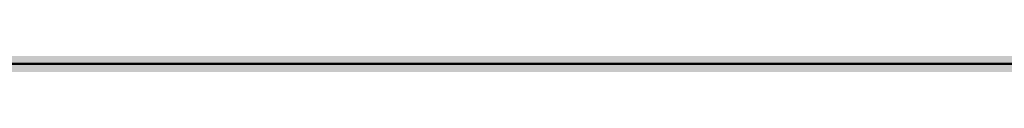
# Model space of a CAD drawing. Units: millimetres. Extents: x 0 to 2267, y 0 to 1823.
# Tile 63 of 256: x 1596.855 to 1600.369, y 1227.247 to 1227.247. Entities that reach past the tile are written whole.
import ezdxf

# ---------------------------------------------------------------- set-up
doc = ezdxf.new("R2010")
doc.units = ezdxf.units.MM
doc.header["$MEASUREMENT"] = 0
doc.layers.add('M-HATC', color=252, linetype='Continuous', lineweight=18)
doc.layers.add('M-OUTL', color=7, linetype='Continuous', lineweight=50)

msp = doc.modelspace()

# ---------------------------------------------------------------- hatches: boundary and pattern name
at = {"layer": 'M-HATC'}
h = msp.add_hatch(color=256, dxfattribs=at)
h.dxf.hatch_style = 1
h.paths.add_polyline_path([(2055.771, 1603.062), (1381.0868, 1603.062), (1381.0868, 1598.062), (2055.771, 1598.062)])
h.paths.add_polyline_path([(2055.771, 1598.062), (1381.0868, 1598.062), (1381.0868, 1593.062), (2055.771, 1593.062)])
h.paths.add_polyline_path([(2051.3074, 1536.7609), (1385.5504, 1536.7609), (1385.5504, 1526.7609), (1387.5504, 1526.7609), (1388.5366, 1525.0528), (1385.3319, 1521.2335), (1385.3319, 1521.2226), (2050.2542, 1522.7491), (2048.3212, 1525.0528), (2049.3074, 1526.7609), (2051.3074, 1526.7609)])
edge = h.paths.add_edge_path()
edge.add_arc((1847.5345, 1379.1492), 135, 222.603061, 222.890851, ccw=False)
edge.add_line((1748.1663, 1287.7656), (1683.0921, 1287.7656))
edge.add_arc((1583.7239, 1379.1492), 135, 317.109149, 317.396939, ccw=False)
edge.add_arc((1678.9686, 1290.6707), 5, 222.8909, 317.1091, ccw=False)
edge.add_arc((1774.2133, 1379.1492), 135, 222.603061, 222.890851, ccw=False)
edge.add_line((1674.8451, 1287.7656), (1609.7709, 1287.7656))
edge.add_arc((1510.4027, 1379.1492), 135, 317.109149, 317.396939, ccw=False)
edge.add_arc((1605.6474, 1290.6707), 5, 222.8909, 317.1091, ccw=False)
edge.add_arc((1700.8921, 1379.1492), 135, 222.603061, 222.890851, ccw=False)
edge.add_line((1601.5239, 1287.7656), (1536.4497, 1287.7656))
edge.add_arc((1437.0815, 1379.1492), 135, 317.109149, 317.396939, ccw=False)
edge.add_arc((1532.3262, 1290.6707), 5, 222.8909, 317.1091, ccw=False)
edge.add_arc((1627.5709, 1379.1492), 135, 222.603061, 222.890851, ccw=False)
edge.add_line((1528.2027, 1287.7656), (1505.9289, 1287.7656))
edge.add_spline(control_points=[(1505.9289, 1287.7656), (1504.2622, 1287.7656), (1504.2622, 1282.7656), (1505.9289, 1282.7656)], knot_values=[0, 0, 0, 0, 5, 5, 5, 5], degree=3, periodic=0)
edge.add_line((1505.9289, 1282.7656), (1930.9289, 1282.7656))
edge.add_spline(control_points=[(1930.9289, 1282.7656), (1932.5956, 1282.7656), (1932.5956, 1287.7656), (1930.9289, 1287.7656)], knot_values=[0, 0, 0, 0, 5, 5, 5, 5], degree=3, periodic=0)
edge.add_line((1930.9289, 1287.7656), (1903.0557, 1287.7656))
edge.add_arc((1803.6875, 1379.1492), 135, 317.109149, 317.396939, ccw=False)
edge.add_arc((1898.9322, 1290.6707), 5, 222.8909, 317.1091, ccw=False)
edge.add_arc((1994.1769, 1379.1492), 135, 222.603061, 222.890851, ccw=False)
edge.add_line((1894.8087, 1287.7656), (1829.7345, 1287.7656))
edge.add_arc((1730.3663, 1379.1492), 135, 317.109149, 317.396939, ccw=False)
edge.add_arc((1825.611, 1290.6707), 5, 222.8909, 317.1091, ccw=False)
edge.add_arc((1920.8557, 1379.1492), 135, 222.603061, 222.890851, ccw=False)
edge.add_line((1821.4875, 1287.7656), (1756.4133, 1287.7656))
edge.add_arc((1657.0451, 1379.1492), 135, 317.109149, 317.396939, ccw=False)
edge.add_arc((1752.2898, 1290.6707), 5, 222.8909, 317.1091, ccw=False)
edge = h.paths.add_edge_path()
edge.add_spline(control_points=[(1843.4289, 1227.2475), (1845.0956, 1227.2475), (1845.0956, 1232.2475), (1843.4289, 1232.2475)], knot_values=[0, 0, 0, 0, 5, 5, 5, 5], degree=3, periodic=0)
edge.add_line((1843.4289, 1232.2475), (1593.4289, 1232.2475))
edge.add_spline(control_points=[(1593.4289, 1232.2475), (1591.7622, 1232.2475), (1591.7622, 1227.2475), (1593.4289, 1227.2475)], knot_values=[0, 0, 0, 0, 5, 5, 5, 5], degree=3, periodic=0)
edge.add_line((1593.4289, 1227.2475), (1843.4289, 1227.2475))
h.paths.add_polyline_path([(1905.9289, 1127.4171), (1530.9289, 1127.4171, 0.414214), (1520.9289, 1117.4171), (1530.9289, 1117.4171), (1915.9289, 1117.4171, 0.414214)])
edge = h.paths.add_edge_path()
edge.add_arc((1397.0858, 1498.4078), 12.7299, 90.78215, 190.87871, ccw=False)
edge.add_line((1396.912, 1511.1365), (1428.0097, 1511.3488))
edge.add_line((1428.0097, 1511.3488), (1433.0097, 1511.3488))
edge.add_line((1433.0097, 1511.3488), (1434.439, 1511.3488))
edge.add_arc((1419.474, 1498.0804), 20, 41.561, 74.08211)
edge.add_line((1424.9592, 1517.3135), (1399.9351, 1517.2561))
edge.add_spline(control_points=[(1399.9307, 1517.2561), (1399.884, 1517.2131), (1399.8328, 1517.1689), (1399.7774, 1517.1236)], knot_values=[11.567499, 11.567499, 11.567499, 11.567499, 11.814249, 11.814249, 11.814249, 11.814249], degree=3, periodic=0)
edge.add_spline(control_points=[(1399.6328, 1517.0099), (1399.5831, 1516.9721), (1399.5307, 1516.9338), (1399.4759, 1516.8947)], knot_values=[11.167718, 11.167718, 11.167718, 11.167718, 11.365188, 11.365188, 11.365188, 11.365188], degree=3, periodic=0)
edge.add_spline(control_points=[(1399.3398, 1516.8001), (1399.1514, 1516.6719), (1398.9384, 1516.5377), (1398.704, 1516.3994)], knot_values=[10.376405, 10.376405, 10.376405, 10.376405, 11.00994, 11.00994, 11.00994, 11.00994], degree=3, periodic=0)
edge.add_spline(control_points=[(1398.6572, 1516.3719), (1398.5789, 1516.326), (1398.4983, 1516.2797), (1398.4155, 1516.2331)], knot_values=[10.125175, 10.125175, 10.125175, 10.125175, 10.334406, 10.334406, 10.334406, 10.334406], degree=3, periodic=0)
edge.add_spline(control_points=[(1398.2642, 1516.1487), (1398.196, 1516.1111), (1398.1263, 1516.0732), (1398.0555, 1516.0351)], knot_values=[9.832246, 9.832246, 9.832246, 9.832246, 9.999658, 9.999658, 9.999658, 9.999658], degree=3, periodic=0)
edge.add_spline(control_points=[(1397.9987, 1516.0048), (1397.7312, 1515.8621), (1397.446, 1515.7171), (1397.1466, 1515.5714)], knot_values=[9.161808, 9.161808, 9.161808, 9.161808, 9.787769, 9.787769, 9.787769, 9.787769], degree=3, periodic=0)
edge.add_spline(control_points=[(1397.1466, 1515.5714), (1396.8418, 1515.423), (1396.5222, 1515.274), (1396.1914, 1515.1262)], knot_values=[8.524455, 8.524455, 8.524455, 8.524455, 9.161808, 9.161808, 9.161808, 9.161808], degree=3, periodic=0)
edge.add_spline(control_points=[(1396.0777, 1515.0756), (1395.9854, 1515.0348), (1395.8922, 1514.994), (1395.7983, 1514.9534)], knot_values=[8.275193, 8.275193, 8.275193, 8.275193, 8.451726, 8.451726, 8.451726, 8.451726], degree=3, periodic=0)
edge.add_spline(control_points=[(1395.6018, 1514.8691), (1395.4997, 1514.8257), (1395.3968, 1514.7824), (1395.2932, 1514.7394)], knot_values=[7.962917, 7.962917, 7.962917, 7.962917, 8.152764, 8.152764, 8.152764, 8.152764], degree=3, periodic=0)
edge.add_spline(control_points=[(1395.2116, 1514.7057), (1394.8278, 1514.5475), (1394.4345, 1514.3929), (1394.0364, 1514.2442)], knot_values=[7.21254, 7.21254, 7.21254, 7.21254, 7.913148, 7.913148, 7.913148, 7.913148], degree=3, periodic=0)
edge.add_spline(control_points=[(1394.0364, 1514.2442), (1393.7076, 1514.1214), (1393.3754, 1514.0027), (1393.0427, 1513.8895)], knot_values=[6.633733, 6.633733, 6.633733, 6.633733, 7.21254, 7.21254, 7.21254, 7.21254], degree=3, periodic=0)
edge.add_spline(control_points=[(1392.8214, 1513.815), (1392.7198, 1513.7812), (1392.6181, 1513.7479), (1392.5166, 1513.7152)], knot_values=[6.328796, 6.328796, 6.328796, 6.328796, 6.505493, 6.505493, 6.505493, 6.505493], degree=3, periodic=0)
edge.add_spline(control_points=[(1392.5166, 1513.7152), (1392.3187, 1513.6515), (1392.1212, 1513.59), (1391.9244, 1513.531)], knot_values=[5.984605, 5.984605, 5.984605, 5.984605, 6.328796, 6.328796, 6.328796, 6.328796], degree=3, periodic=0)
edge.add_spline(control_points=[(1391.7915, 1513.4915), (1391.3122, 1513.3501), (1390.8384, 1513.2239), (1390.3784, 1513.1171)], knot_values=[5.066697, 5.066697, 5.066697, 5.066697, 5.907055, 5.907055, 5.907055, 5.907055], degree=3, periodic=0)
edge.add_spline(control_points=[(1390.3784, 1513.1171), (1390.1797, 1513.071), (1389.9836, 1513.0284), (1389.7907, 1512.9899)], knot_values=[4.70367, 4.70367, 4.70367, 4.70367, 5.066695, 5.066695, 5.066695, 5.066695], degree=3, periodic=0)
edge.add_spline(control_points=[(1389.422, 1512.9204), (1389.2459, 1512.8892), (1389.0729, 1512.8617), (1388.9036, 1512.8381)], knot_values=[4.130571, 4.130571, 4.130571, 4.130571, 4.469816, 4.469816, 4.469816, 4.469816], degree=3, periodic=0)
edge.add_spline(control_points=[(1388.9036, 1512.8381), (1388.591, 1512.7946), (1388.2911, 1512.7644), (1388.0071, 1512.7494)], knot_values=[3.504031, 3.504031, 3.504031, 3.504031, 4.130571, 4.130571, 4.130571, 4.130571], degree=3, periodic=0)
edge.add_spline(control_points=[(1387.9356, 1512.7459), (1387.8538, 1512.7423), (1387.7733, 1512.74), (1387.6944, 1512.739)], knot_values=[3.268866, 3.268866, 3.268866, 3.268866, 3.451164, 3.451164, 3.451164, 3.451164], degree=3, periodic=0)
edge.add_spline(control_points=[(1387.3351, 1512.7443), (1387.2076, 1512.7499), (1387.0847, 1512.7597), (1386.967, 1512.7739)], knot_values=[2.670686, 2.670686, 2.670686, 2.670686, 2.984, 2.984, 2.984, 2.984], degree=3, periodic=0)
edge.add_spline(control_points=[(1386.8327, 1512.7922), (1386.8209, 1512.7941), (1386.8092, 1512.7959), (1386.7975, 1512.7979)], knot_values=[2.516981, 2.516981, 2.516981, 2.516981, 2.549528, 2.549528, 2.549528, 2.549528], degree=3, periodic=0)
edge.add_spline(control_points=[(1386.4526, 1512.8735), (1386.4257, 1512.881), (1386.3993, 1512.889), (1386.3733, 1512.8972)], knot_values=[2.095869, 2.095869, 2.095869, 2.095869, 2.17941, 2.17941, 2.17941, 2.17941], degree=3, periodic=0)
edge.add_spline(control_points=[(1386.0691, 1513.0189), (1386.0634, 1513.0217), (1386.0577, 1513.0246), (1386.052, 1513.0275)], knot_values=[1.72453, 1.72453, 1.72453, 1.72453, 1.745933, 1.745933, 1.745933, 1.745933], degree=3, periodic=0)
edge.add_arc((1399.474, 1498.0804), 20, 131.82432, 180)
edge.add_arc((1630.3336, 1505.5484), 250.9708, 181.705176, 236.427975)
edge.add_arc((1605.3399, 1483.3044), 218.7822, 238.660829, 243.34961)
edge.add_arc((1647.0911, 1510.3592), 262.8986, 183.129836, 237.853442, ccw=False)
h.paths.add_polyline_path([(1406.5369, 1391.9644, 0.149382), (1491.5506, 1296.4418, -0.129517)], flags=17)
edge = h.paths.add_edge_path()
edge.add_arc((2037.3838, 1498.0804), 20, 0, 48.26587)
edge.add_spline(control_points=[(2050.6973, 1513.0052), (2050.6512, 1512.9847), (2050.6034, 1512.9655), (2050.5539, 1512.9477)], knot_values=[1.835652, 1.835652, 1.835652, 1.835652, 2.000781, 2.000781, 2.000781, 2.000781], degree=3, periodic=0)
edge.add_spline(control_points=[(2050.4616, 1512.9166), (2050.479, 1512.9221), (2050.4963, 1512.9277), (2050.5133, 1512.9335)], knot_values=[2.045477, 2.045477, 2.045477, 2.045477, 2.101389, 2.101389, 2.101389, 2.101389], degree=3, periodic=0)
edge.add_spline(control_points=[(2050.129, 1512.8342), (2050.1984, 1512.8473), (2050.2657, 1512.8623), (2050.3308, 1512.8792)], knot_values=[2.237629, 2.237629, 2.237629, 2.237629, 2.435841, 2.435841, 2.435841, 2.435841], degree=3, periodic=0)
edge.add_spline(control_points=[(2050.0946, 1512.8278), (2050.1061, 1512.8299), (2050.1176, 1512.832), (2050.129, 1512.8342)], knot_values=[2.435841, 2.435841, 2.435841, 2.435841, 2.468321, 2.468321, 2.468321, 2.468321], degree=3, periodic=0)
edge.add_spline(control_points=[(2049.7843, 1512.7851), (2049.8552, 1512.7922), (2049.9243, 1512.8008), (2049.9917, 1512.8109)], knot_values=[2.563852, 2.563852, 2.563852, 2.563852, 2.748541, 2.748541, 2.748541, 2.748541], degree=3, periodic=0)
edge.add_spline(control_points=[(2049.4052, 1512.7617), (2049.5364, 1512.7653), (2049.6629, 1512.773), (2049.7843, 1512.7851)], knot_values=[2.748541, 2.748541, 2.748541, 2.748541, 3.064882, 3.064882, 3.064882, 3.064882], degree=3, periodic=0)
edge.add_spline(control_points=[(2049.1698, 1512.7597), (2049.2336, 1512.7591), (2049.2965, 1512.7594), (2049.3584, 1512.7606)], knot_values=[3.102309, 3.102309, 3.102309, 3.102309, 3.2503, 3.2503, 3.2503, 3.2503], degree=3, periodic=0)
edge.add_spline(control_points=[(2048.8573, 1512.7691), (2048.9638, 1512.7638), (2049.068, 1512.7606), (2049.1698, 1512.7597)], knot_values=[3.2503, 3.2503, 3.2503, 3.2503, 3.486069, 3.486069, 3.486069, 3.486069], degree=3, periodic=0)
edge.add_spline(control_points=[(2048.6924, 1512.7789), (2048.3729, 1512.8009), (2048.0345, 1512.8411), (2047.6817, 1512.897)], knot_values=[3.606429, 3.606429, 3.606429, 3.606429, 4.2989, 4.2989, 4.2989, 4.2989], degree=3, periodic=0)
edge.add_spline(control_points=[(2047.6817, 1512.897), (2047.5458, 1512.9185), (2047.4077, 1512.9424), (2047.2678, 1512.9685)], knot_values=[4.2989, 4.2989, 4.2989, 4.2989, 4.565769, 4.565769, 4.565769, 4.565769], degree=3, periodic=0)
edge.add_spline(control_points=[(2047.2678, 1512.9685), (2047.1449, 1512.9914), (2047.0207, 1513.016), (2046.8951, 1513.0422)], knot_values=[4.565769, 4.565769, 4.565769, 4.565769, 4.799971, 4.799971, 4.799971, 4.799971], degree=3, periodic=0)
edge.add_spline(control_points=[(2046.8951, 1513.0422), (2046.5286, 1513.1188), (2046.1513, 1513.209), (2045.7676, 1513.3107)], knot_values=[4.799971, 4.799971, 4.799971, 4.799971, 5.483718, 5.483718, 5.483718, 5.483718], degree=3, periodic=0)
edge.add_spline(control_points=[(2045.7676, 1513.3107), (2045.3724, 1513.4154), (2044.9704, 1513.5322), (2044.5662, 1513.6588)], knot_values=[5.483718, 5.483718, 5.483718, 5.483718, 6.187866, 6.187866, 6.187866, 6.187866], degree=3, periodic=0)
edge.add_spline(control_points=[(2044.5662, 1513.6588), (2044.4149, 1513.7061), (2044.2633, 1513.7549), (2044.1116, 1513.8048)], knot_values=[6.187866, 6.187866, 6.187866, 6.187866, 6.451551, 6.451551, 6.451551, 6.451551], degree=3, periodic=0)
edge.add_spline(control_points=[(2044.1116, 1513.8048), (2043.9967, 1513.8427), (2043.8817, 1513.8813), (2043.7668, 1513.9205)], knot_values=[6.451551, 6.451551, 6.451551, 6.451551, 6.651434, 6.651434, 6.651434, 6.651434], degree=3, periodic=0)
edge.add_spline(control_points=[(2043.7668, 1513.9205), (2043.3716, 1514.0554), (2042.9774, 1514.1979), (2042.5886, 1514.3458)], knot_values=[6.651434, 6.651434, 6.651434, 6.651434, 7.338879, 7.338879, 7.338879, 7.338879], degree=3, periodic=0)
edge.add_spline(control_points=[(2042.5886, 1514.3458), (2042.1643, 1514.5071), (2041.7465, 1514.6749), (2041.3409, 1514.846)], knot_values=[7.338879, 7.338879, 7.338879, 7.338879, 8.089209, 8.089209, 8.089209, 8.089209], degree=3, periodic=0)
edge.add_spline(control_points=[(2041.3409, 1514.846), (2041.1028, 1514.9465), (2040.869, 1515.0481), (2040.6405, 1515.1502)], knot_values=[8.089209, 8.089209, 8.089209, 8.089209, 8.529587, 8.529587, 8.529587, 8.529587], degree=3, periodic=0)
edge.add_spline(control_points=[(2040.51, 1515.2089), (2040.0824, 1515.4022), (2039.6747, 1515.5971), (2039.295, 1515.7894)], knot_values=[8.613818, 8.613818, 8.613818, 8.613818, 9.44571, 9.44571, 9.44571, 9.44571], degree=3, periodic=0)
edge.add_spline(control_points=[(2039.295, 1515.7894), (2039.0618, 1515.9075), (2038.8391, 1516.0246), (2038.6288, 1516.1398)], knot_values=[9.44571, 9.44571, 9.44571, 9.44571, 9.956404, 9.956404, 9.956404, 9.956404], degree=3, periodic=0)
edge.add_spline(control_points=[(2038.6288, 1516.1398), (2038.5187, 1516.2001), (2038.4121, 1516.2598), (2038.309, 1516.3189)], knot_values=[9.956404, 9.956404, 9.956404, 9.956404, 10.223542, 10.223542, 10.223542, 10.223542], degree=3, periodic=0)
edge.add_spline(control_points=[(2038.309, 1516.3189), (2038.2138, 1516.3735), (2038.1216, 1516.4276), (2038.0328, 1516.481)], knot_values=[10.223542, 10.223542, 10.223542, 10.223542, 10.47051, 10.47051, 10.47051, 10.47051], degree=3, periodic=0)
edge.add_spline(control_points=[(2038.0328, 1516.481), (2037.7855, 1516.6296), (2037.5639, 1516.773), (2037.3722, 1516.909)], knot_values=[10.47051, 10.47051, 10.47051, 10.47051, 11.15767, 11.15767, 11.15767, 11.15767], degree=3, periodic=0)
edge.add_spline(control_points=[(2037.3722, 1516.909), (2037.2789, 1516.9752), (2037.1927, 1517.0396), (2037.1142, 1517.102)], knot_values=[11.15767, 11.15767, 11.15767, 11.15767, 11.49227, 11.49227, 11.49227, 11.49227], degree=3, periodic=0)
edge.add_spline(control_points=[(2036.8564, 1517.3259), (2036.9148, 1517.2692), (2036.9814, 1517.2103), (2037.0557, 1517.1492)], knot_values=[11.577341, 11.577341, 11.577341, 11.577341, 11.91035, 11.91035, 11.91035, 11.91035], degree=3, periodic=0)
edge.add_spline(control_points=[(2036.8074, 1517.3748), (2036.823, 1517.3587), (2036.8393, 1517.3424), (2036.8564, 1517.3259)], knot_values=[11.91035, 11.91035, 11.91035, 11.91035, 12.007402, 12.007402, 12.007402, 12.007402], degree=3, periodic=0)
edge.add_spline(control_points=[(2036.7017, 1517.494), (2036.7104, 1517.483), (2036.7196, 1517.4719), (2036.7291, 1517.4606)], knot_values=[12.184155, 12.184155, 12.184155, 12.184155, 12.255409, 12.255409, 12.255409, 12.255409], degree=3, periodic=0)
edge.add_spline(control_points=[(2036.6159, 1517.6205), (2036.62, 1517.613), (2036.6243, 1517.6055), (2036.6289, 1517.5979)], knot_values=[12.487913, 12.487913, 12.487913, 12.487913, 12.541035, 12.541035, 12.541035, 12.541035], degree=3, periodic=0)
edge.add_spline(control_points=[(2036.5635, 1517.786), (2036.5637, 1517.7794), (2036.5642, 1517.7726), (2036.565, 1517.7658)], knot_values=[12.911761, 12.911761, 12.911761, 12.911761, 12.968286, 12.968286, 12.968286, 12.968286], degree=3, periodic=0)
edge.add_spline(control_points=[(2036.6166, 1517.9304), (2036.6125, 1517.9259), (2036.6086, 1517.9212), (2036.6049, 1517.9165)], knot_values=[13.382527, 13.382527, 13.382527, 13.382527, 13.433791, 13.433791, 13.433791, 13.433791], degree=3, periodic=0)
edge.add_spline(control_points=[(2036.749, 1518.017), (2036.7361, 1518.0116), (2036.7239, 1518.006), (2036.7124, 1518.0002)], knot_values=[13.726299, 13.726299, 13.726299, 13.726299, 13.809928, 13.809928, 13.809928, 13.809928], degree=3, periodic=0)
edge.add_spline(control_points=[(2036.8604, 1518.0528), (2036.8386, 1518.0474), (2036.8181, 1518.0416), (2036.7988, 1518.0353)], knot_values=[13.910887, 13.910887, 13.910887, 13.910887, 14.02153, 14.02153, 14.02153, 14.02153], degree=3, periodic=0)
edge.add_line((2036.9639, 1518.0804), (2032.3838, 1518.0804))
edge.add_line((2032.3838, 1518.0804), (2027.3838, 1518.0804))
edge.add_line((2027.3838, 1518.0804), (2022.3838, 1518.0804))
edge.add_line((2022.3838, 1518.0804), (2017.3838, 1518.0804))
edge.add_arc((2017.3838, 1498.0804), 20, 90, 138.439)
edge.add_line((2002.4188, 1511.3488), (2003.8481, 1511.3488))
edge.add_line((2003.8481, 1511.3488), (2008.8481, 1511.3488))
edge.add_line((2008.8481, 1511.3488), (2039.772, 1511.1377))
edge.add_arc((2039.772, 1498.4078), 12.7299, -10.87871, 90, ccw=False)
edge.add_arc((1789.7668, 1510.3592), 262.8986, 302.146558, 356.870164, ccw=False)
edge.add_arc((1831.5179, 1483.3044), 218.7822, 296.65039, 301.339171)
edge.add_arc((1806.5242, 1505.5484), 250.9708, 303.572025, 358.294824)
h.paths.add_polyline_path([(2030.321, 1391.9644, -0.129517), (1945.3072, 1296.4418, 0.149382)], flags=17)
edge = h.paths.add_edge_path()
edge.add_spline(control_points=[(2037.2464, 1518.0821), (2037.2898, 1518.081), (2037.3355, 1518.0804), (2037.3838, 1518.0804)], knot_values=[0.000012, 0.000012, 0.000012, 0.000012, 0.144754, 0.144754, 0.144754, 0.144754], degree=3, periodic=0)
edge.add_line((2037.3357, 1518.0804), (2037.0096, 1518.0804))
edge.add_spline(control_points=[(2037.0096, 1518.0804), (2036.9822, 1518.0768), (2036.956, 1518.0727), (2036.9312, 1518.0681)], knot_values=[14.13465, 14.13465, 14.13465, 14.13465, 14.247197, 14.247197, 14.247197, 14.247197], degree=3, periodic=0)
edge.add_spline(control_points=[(2036.9312, 1518.0681), (2036.9276, 1518.0674), (2036.9241, 1518.0667), (2036.9205, 1518.0661)], knot_values=[14.118315, 14.118315, 14.118315, 14.118315, 14.13465, 14.13465, 14.13465, 14.13465], degree=3, periodic=0)
edge.add_spline(control_points=[(2036.9205, 1518.0661), (2036.9118, 1518.0644), (2036.9032, 1518.0626), (2036.8948, 1518.0608)], knot_values=[14.078086, 14.078086, 14.078086, 14.078086, 14.118315, 14.118315, 14.118315, 14.118315], degree=3, periodic=0)
edge.add_spline(control_points=[(2036.8948, 1518.0608), (2036.883, 1518.0583), (2036.8716, 1518.0556), (2036.8604, 1518.0528)], knot_values=[14.02153, 14.02153, 14.02153, 14.02153, 14.078086, 14.078086, 14.078086, 14.078086], degree=3, periodic=0)
edge.add_spline(control_points=[(2036.8604, 1518.0528), (2036.8386, 1518.0474), (2036.8181, 1518.0416), (2036.7988, 1518.0353)], knot_values=[13.910887, 13.910887, 13.910887, 13.910887, 14.02153, 14.02153, 14.02153, 14.02153], degree=3, periodic=0)
edge.add_spline(control_points=[(2036.7988, 1518.0353), (2036.7981, 1518.035), (2036.7974, 1518.0348), (2036.7967, 1518.0346)], knot_values=[13.906906, 13.906906, 13.906906, 13.906906, 13.910887, 13.910887, 13.910887, 13.910887], degree=3, periodic=0)
edge.add_spline(control_points=[(2036.7967, 1518.0346), (2036.7882, 1518.0318), (2036.7799, 1518.0289), (2036.7719, 1518.0259)], knot_values=[13.857826, 13.857826, 13.857826, 13.857826, 13.906906, 13.906906, 13.906906, 13.906906], degree=3, periodic=0)
edge.add_spline(control_points=[(2036.7719, 1518.0259), (2036.764, 1518.023), (2036.7564, 1518.02), (2036.749, 1518.017)], knot_values=[13.809928, 13.809928, 13.809928, 13.809928, 13.857826, 13.857826, 13.857826, 13.857826], degree=3, periodic=0)
edge.add_spline(control_points=[(2036.749, 1518.017), (2036.7361, 1518.0116), (2036.7239, 1518.006), (2036.7124, 1518.0002)], knot_values=[13.726299, 13.726299, 13.726299, 13.726299, 13.809928, 13.809928, 13.809928, 13.809928], degree=3, periodic=0)
edge.add_spline(control_points=[(2036.7124, 1518.0002), (2036.7121, 1518), (2036.7118, 1517.9999), (2036.7115, 1517.9997)], knot_values=[13.723993, 13.723993, 13.723993, 13.723993, 13.726299, 13.726299, 13.726299, 13.726299], degree=3, periodic=0)
edge.add_spline(control_points=[(2036.7115, 1517.9997), (2036.7063, 1517.9971), (2036.7013, 1517.9944), (2036.6965, 1517.9917)], knot_values=[13.686536, 13.686536, 13.686536, 13.686536, 13.723993, 13.723993, 13.723993, 13.723993], degree=3, periodic=0)
edge.add_spline(control_points=[(2036.6965, 1517.9917), (2036.6919, 1517.9891), (2036.6874, 1517.9865), (2036.6831, 1517.9839)], knot_values=[13.651251, 13.651251, 13.651251, 13.651251, 13.686536, 13.686536, 13.686536, 13.686536], degree=3, periodic=0)
edge.add_spline(control_points=[(2036.6831, 1517.9839), (2036.6764, 1517.9798), (2036.67, 1517.9757), (2036.6639, 1517.9714)], knot_values=[13.596804, 13.596804, 13.596804, 13.596804, 13.651251, 13.651251, 13.651251, 13.651251], degree=3, periodic=0)
edge.add_spline(control_points=[(2036.6639, 1517.9714), (2036.6636, 1517.9712), (2036.6633, 1517.9709), (2036.6629, 1517.9707)], knot_values=[13.593956, 13.593956, 13.593956, 13.593956, 13.596804, 13.596804, 13.596804, 13.596804], degree=3, periodic=0)
edge.add_spline(control_points=[(2036.6629, 1517.9707), (2036.6603, 1517.9689), (2036.6577, 1517.967), (2036.6552, 1517.9651)], knot_values=[13.570322, 13.570322, 13.570322, 13.570322, 13.593956, 13.593956, 13.593956, 13.593956], degree=3, periodic=0)
edge.add_spline(control_points=[(2036.6552, 1517.9651), (2036.6525, 1517.9631), (2036.6499, 1517.9611), (2036.6474, 1517.9591)], knot_values=[13.545477, 13.545477, 13.545477, 13.545477, 13.570322, 13.570322, 13.570322, 13.570322], degree=3, periodic=0)
edge.add_spline(control_points=[(2036.6474, 1517.9591), (2036.6472, 1517.9589), (2036.6471, 1517.9588), (2036.6469, 1517.9587)], knot_values=[13.543931, 13.543931, 13.543931, 13.543931, 13.545477, 13.545477, 13.545477, 13.545477], degree=3, periodic=0)
edge.add_spline(control_points=[(2036.6469, 1517.9587), (2036.6412, 1517.9541), (2036.6358, 1517.9494), (2036.6307, 1517.9447)], knot_values=[13.488237, 13.488237, 13.488237, 13.488237, 13.543931, 13.543931, 13.543931, 13.543931], degree=3, periodic=0)
edge.add_spline(control_points=[(2036.6307, 1517.9447), (2036.6282, 1517.9423), (2036.6257, 1517.9399), (2036.6233, 1517.9374)], knot_values=[13.460307, 13.460307, 13.460307, 13.460307, 13.488237, 13.488237, 13.488237, 13.488237], degree=3, periodic=0)
edge.add_spline(control_points=[(2036.6233, 1517.9374), (2036.6215, 1517.9356), (2036.6198, 1517.9338), (2036.6181, 1517.932)], knot_values=[13.439712, 13.439712, 13.439712, 13.439712, 13.460307, 13.460307, 13.460307, 13.460307], degree=3, periodic=0)
edge.add_spline(control_points=[(2036.6181, 1517.932), (2036.6176, 1517.9315), (2036.6171, 1517.9309), (2036.6166, 1517.9304)], knot_values=[13.433791, 13.433791, 13.433791, 13.433791, 13.439712, 13.439712, 13.439712, 13.439712], degree=3, periodic=0)
edge.add_spline(control_points=[(2036.6166, 1517.9304), (2036.6125, 1517.9259), (2036.6086, 1517.9212), (2036.6049, 1517.9165)], knot_values=[13.382527, 13.382527, 13.382527, 13.382527, 13.433791, 13.433791, 13.433791, 13.433791], degree=3, periodic=0)
edge.add_spline(control_points=[(2036.6049, 1517.9165), (2036.6026, 1517.9135), (2036.6004, 1517.9104), (2036.5982, 1517.9074)], knot_values=[13.350017, 13.350017, 13.350017, 13.350017, 13.382527, 13.382527, 13.382527, 13.382527], degree=3, periodic=0)
edge.add_spline(control_points=[(2036.5982, 1517.9074), (2036.5972, 1517.9059), (2036.5962, 1517.9043), (2036.5952, 1517.9028)], knot_values=[13.333922, 13.333922, 13.333922, 13.333922, 13.350017, 13.350017, 13.350017, 13.350017], degree=3, periodic=0)
edge.add_spline(control_points=[(2036.5952, 1517.9028), (2036.5945, 1517.9018), (2036.5939, 1517.9009), (2036.5933, 1517.8999)], knot_values=[13.323828, 13.323828, 13.323828, 13.323828, 13.333922, 13.333922, 13.333922, 13.333922], degree=3, periodic=0)
edge.add_spline(control_points=[(2036.5933, 1517.8999), (2036.5905, 1517.8955), (2036.5879, 1517.8909), (2036.5855, 1517.8864)], knot_values=[13.277545, 13.277545, 13.277545, 13.277545, 13.323828, 13.323828, 13.323828, 13.323828], degree=3, periodic=0)
edge.add_spline(control_points=[(2036.5855, 1517.8864), (2036.5836, 1517.8827), (2036.5817, 1517.8789), (2036.5801, 1517.8751)], knot_values=[13.240119, 13.240119, 13.240119, 13.240119, 13.277545, 13.277545, 13.277545, 13.277545], degree=3, periodic=0)
edge.add_spline(control_points=[(2036.5801, 1517.8751), (2036.5795, 1517.8739), (2036.579, 1517.8727), (2036.5785, 1517.8715)], knot_values=[13.228211, 13.228211, 13.228211, 13.228211, 13.240119, 13.240119, 13.240119, 13.240119], degree=3, periodic=0)
edge.add_spline(control_points=[(2036.5785, 1517.8715), (2036.578, 1517.8702), (2036.5774, 1517.869), (2036.5769, 1517.8677)], knot_values=[13.215717, 13.215717, 13.215717, 13.215717, 13.228211, 13.228211, 13.228211, 13.228211], degree=3, periodic=0)
edge.add_spline(control_points=[(2036.5769, 1517.8677), (2036.5755, 1517.864), (2036.5741, 1517.8603), (2036.5729, 1517.8565)], knot_values=[13.179847, 13.179847, 13.179847, 13.179847, 13.215717, 13.215717, 13.215717, 13.215717], degree=3, periodic=0)
edge.add_spline(control_points=[(2036.5729, 1517.8565), (2036.5713, 1517.8515), (2036.5699, 1517.8464), (2036.5687, 1517.8413)], knot_values=[13.132017, 13.132017, 13.132017, 13.132017, 13.179847, 13.179847, 13.179847, 13.179847], degree=3, periodic=0)
edge.add_spline(control_points=[(2036.5687, 1517.8413), (2036.5684, 1517.8402), (2036.5682, 1517.8392), (2036.568, 1517.8382)], knot_values=[13.122482, 13.122482, 13.122482, 13.122482, 13.132017, 13.132017, 13.132017, 13.132017], degree=3, periodic=0)
edge.add_spline(control_points=[(2036.568, 1517.8382), (2036.5676, 1517.8363), (2036.5672, 1517.8345), (2036.5669, 1517.8327)], knot_values=[13.105592, 13.105592, 13.105592, 13.105592, 13.122482, 13.122482, 13.122482, 13.122482], degree=3, periodic=0)
edge.add_spline(control_points=[(2036.5669, 1517.8327), (2036.5662, 1517.8292), (2036.5657, 1517.8257), (2036.5652, 1517.8222)], knot_values=[13.074063, 13.074063, 13.074063, 13.074063, 13.105592, 13.105592, 13.105592, 13.105592], degree=3, periodic=0)
edge.add_spline(control_points=[(2036.5652, 1517.8222), (2036.5652, 1517.8222), (2036.5652, 1517.8222), (2036.5652, 1517.8222)], knot_values=[13.074043, 13.074043, 13.074043, 13.074043, 13.074063, 13.074063, 13.074063, 13.074063], degree=3, periodic=0)
edge.add_spline(control_points=[(2036.5652, 1517.8222), (2036.5644, 1517.8164), (2036.5639, 1517.8106), (2036.5636, 1517.8046)], knot_values=[13.021884, 13.021884, 13.021884, 13.021884, 13.074043, 13.074043, 13.074043, 13.074043], degree=3, periodic=0)
edge.add_spline(control_points=[(2036.5636, 1517.8046), (2036.5636, 1517.804), (2036.5636, 1517.8034), (2036.5635, 1517.8028)], knot_values=[13.01674, 13.01674, 13.01674, 13.01674, 13.021884, 13.021884, 13.021884, 13.021884], degree=3, periodic=0)
edge.add_spline(control_points=[(2036.5635, 1517.8028), (2036.5634, 1517.8005), (2036.5634, 1517.7982), (2036.5634, 1517.7958)], knot_values=[12.996438, 12.996438, 12.996438, 12.996438, 13.01674, 13.01674, 13.01674, 13.01674], degree=3, periodic=0)
edge.add_spline(control_points=[(2036.5634, 1517.7958), (2036.5633, 1517.7926), (2036.5634, 1517.7893), (2036.5635, 1517.786)], knot_values=[12.968286, 12.968286, 12.968286, 12.968286, 12.996438, 12.996438, 12.996438, 12.996438], degree=3, periodic=0)
edge.add_spline(control_points=[(2036.5635, 1517.786), (2036.5637, 1517.7794), (2036.5642, 1517.7726), (2036.565, 1517.7658)], knot_values=[12.911761, 12.911761, 12.911761, 12.911761, 12.968286, 12.968286, 12.968286, 12.968286], degree=3, periodic=0)
edge.add_spline(control_points=[(2036.565, 1517.7658), (2036.565, 1517.7657), (2036.565, 1517.7656), (2036.565, 1517.7656)], knot_values=[12.911017, 12.911017, 12.911017, 12.911017, 12.911761, 12.911761, 12.911761, 12.911761], degree=3, periodic=0)
edge.add_spline(control_points=[(2036.565, 1517.7656), (2036.5654, 1517.7625), (2036.5658, 1517.7593), (2036.5663, 1517.7562)], knot_values=[12.88528, 12.88528, 12.88528, 12.88528, 12.911017, 12.911017, 12.911017, 12.911017], degree=3, periodic=0)
edge.add_spline(control_points=[(2036.5663, 1517.7562), (2036.5667, 1517.7534), (2036.5672, 1517.7506), (2036.5677, 1517.7478)], knot_values=[12.862519, 12.862519, 12.862519, 12.862519, 12.88528, 12.88528, 12.88528, 12.88528], degree=3, periodic=0)
edge.add_spline(control_points=[(2036.5677, 1517.7478), (2036.5678, 1517.7474), (2036.5679, 1517.7469), (2036.568, 1517.7465)], knot_values=[12.858885, 12.858885, 12.858885, 12.858885, 12.862519, 12.862519, 12.862519, 12.862519], degree=3, periodic=0)
edge.add_spline(control_points=[(2036.568, 1517.7465), (2036.5692, 1517.7399), (2036.5707, 1517.7332), (2036.5724, 1517.7264)], knot_values=[12.8053, 12.8053, 12.8053, 12.8053, 12.858885, 12.858885, 12.858885, 12.858885], degree=3, periodic=0)
edge.add_spline(control_points=[(2036.5724, 1517.7264), (2036.5734, 1517.7226), (2036.5745, 1517.7187), (2036.5756, 1517.7149)], knot_values=[12.775176, 12.775176, 12.775176, 12.775176, 12.8053, 12.8053, 12.8053, 12.8053], degree=3, periodic=0)
edge.add_spline(control_points=[(2036.5756, 1517.7149), (2036.5763, 1517.7125), (2036.577, 1517.7102), (2036.5778, 1517.7078)], knot_values=[12.756759, 12.756759, 12.756759, 12.756759, 12.775176, 12.775176, 12.775176, 12.775176], degree=3, periodic=0)
edge.add_spline(control_points=[(2036.5778, 1517.7078), (2036.5781, 1517.7067), (2036.5784, 1517.7057), (2036.5787, 1517.7047)], knot_values=[12.748742, 12.748742, 12.748742, 12.748742, 12.756759, 12.756759, 12.756759, 12.756759], degree=3, periodic=0)
edge.add_spline(control_points=[(2036.5787, 1517.7047), (2036.5808, 1517.6983), (2036.5831, 1517.6919), (2036.5856, 1517.6854)], knot_values=[12.69959, 12.69959, 12.69959, 12.69959, 12.748742, 12.748742, 12.748742, 12.748742], degree=3, periodic=0)
edge.add_spline(control_points=[(2036.5856, 1517.6854), (2036.5876, 1517.68), (2036.5898, 1517.6746), (2036.5921, 1517.6692)], knot_values=[12.659038, 12.659038, 12.659038, 12.659038, 12.69959, 12.69959, 12.69959, 12.69959], degree=3, periodic=0)
edge.add_spline(control_points=[(2036.5921, 1517.6692), (2036.594, 1517.6648), (2036.5959, 1517.6605), (2036.5979, 1517.6561)], knot_values=[12.626806, 12.626806, 12.626806, 12.626806, 12.659038, 12.659038, 12.659038, 12.659038], degree=3, periodic=0)
edge.add_spline(control_points=[(2036.5979, 1517.6561), (2036.5984, 1517.6551), (2036.5989, 1517.6541), (2036.5993, 1517.6531)], knot_values=[12.619394, 12.619394, 12.619394, 12.619394, 12.626806, 12.626806, 12.626806, 12.626806], degree=3, periodic=0)
edge.add_spline(control_points=[(2036.5993, 1517.6531), (2036.6043, 1517.6424), (2036.6099, 1517.6315), (2036.6159, 1517.6205)], knot_values=[12.541039, 12.541039, 12.541039, 12.541039, 12.619394, 12.619394, 12.619394, 12.619394], degree=3, periodic=0)
edge.add_spline(control_points=[(2036.6159, 1517.6205), (2036.6159, 1517.6205), (2036.6159, 1517.6205), (2036.6159, 1517.6205)], knot_values=[12.541035, 12.541035, 12.541035, 12.541035, 12.541039, 12.541039, 12.541039, 12.541039], degree=3, periodic=0)
edge.add_spline(control_points=[(2036.6159, 1517.6205), (2036.62, 1517.613), (2036.6243, 1517.6055), (2036.6289, 1517.5979)], knot_values=[12.487913, 12.487913, 12.487913, 12.487913, 12.541035, 12.541035, 12.541035, 12.541035], degree=3, periodic=0)
edge.add_spline(control_points=[(2036.6289, 1517.5979), (2036.6326, 1517.5916), (2036.6365, 1517.5853), (2036.6406, 1517.5789)], knot_values=[12.443982, 12.443982, 12.443982, 12.443982, 12.487913, 12.487913, 12.487913, 12.487913], degree=3, periodic=0)
edge.add_spline(control_points=[(2036.6406, 1517.5789), (2036.6414, 1517.5776), (2036.6423, 1517.5763), (2036.6431, 1517.5749)], knot_values=[12.434996, 12.434996, 12.434996, 12.434996, 12.443982, 12.443982, 12.443982, 12.443982], degree=3, periodic=0)
edge.add_spline(control_points=[(2036.6431, 1517.5749), (2036.6531, 1517.5596), (2036.6639, 1517.5439), (2036.6756, 1517.528)], knot_values=[12.329647, 12.329647, 12.329647, 12.329647, 12.434996, 12.434996, 12.434996, 12.434996], degree=3, periodic=0)
edge.add_spline(control_points=[(2036.6756, 1517.528), (2036.6839, 1517.5168), (2036.6925, 1517.5055), (2036.7017, 1517.494)], knot_values=[12.255409, 12.255409, 12.255409, 12.255409, 12.329647, 12.329647, 12.329647, 12.329647], degree=3, periodic=0)
edge.add_spline(control_points=[(2036.7017, 1517.494), (2036.7104, 1517.483), (2036.7196, 1517.4719), (2036.7291, 1517.4606)], knot_values=[12.184155, 12.184155, 12.184155, 12.184155, 12.255409, 12.255409, 12.255409, 12.255409], degree=3, periodic=0)
edge.add_spline(control_points=[(2036.7291, 1517.4606), (2036.7436, 1517.4435), (2036.759, 1517.4262), (2036.7753, 1517.4085)], knot_values=[12.075961, 12.075961, 12.075961, 12.075961, 12.184155, 12.184155, 12.184155, 12.184155], degree=3, periodic=0)
edge.add_spline(control_points=[(2036.7753, 1517.4085), (2036.7763, 1517.4075), (2036.7773, 1517.4064), (2036.7783, 1517.4054)], knot_values=[12.069502, 12.069502, 12.069502, 12.069502, 12.075961, 12.075961, 12.075961, 12.075961], degree=3, periodic=0)
edge.add_spline(control_points=[(2036.7783, 1517.4054), (2036.7877, 1517.3953), (2036.7974, 1517.385), (2036.8074, 1517.3748)], knot_values=[12.007402, 12.007402, 12.007402, 12.007402, 12.069502, 12.069502, 12.069502, 12.069502], degree=3, periodic=0)
edge.add_spline(control_points=[(2036.8074, 1517.3748), (2036.823, 1517.3587), (2036.8393, 1517.3424), (2036.8564, 1517.3259)], knot_values=[11.91035, 11.91035, 11.91035, 11.91035, 12.007402, 12.007402, 12.007402, 12.007402], degree=3, periodic=0)
edge.add_spline(control_points=[(2036.8564, 1517.3259), (2036.9148, 1517.2692), (2036.9814, 1517.2103), (2037.0557, 1517.1492)], knot_values=[11.577341, 11.577341, 11.577341, 11.577341, 11.91035, 11.91035, 11.91035, 11.91035], degree=3, periodic=0)
edge.add_spline(control_points=[(2037.0557, 1517.1492), (2037.0747, 1517.1336), (2037.0942, 1517.1179), (2037.1142, 1517.102)], knot_values=[11.49227, 11.49227, 11.49227, 11.49227, 11.577341, 11.577341, 11.577341, 11.577341], degree=3, periodic=0)
edge.add_spline(control_points=[(2037.1142, 1517.102), (2037.1927, 1517.0396), (2037.2789, 1516.9752), (2037.3722, 1516.909)], knot_values=[11.15767, 11.15767, 11.15767, 11.15767, 11.49227, 11.49227, 11.49227, 11.49227], degree=3, periodic=0)
edge.add_spline(control_points=[(2037.3722, 1516.909), (2037.5639, 1516.773), (2037.7855, 1516.6296), (2038.0328, 1516.481)], knot_values=[10.47051, 10.47051, 10.47051, 10.47051, 11.15767, 11.15767, 11.15767, 11.15767], degree=3, periodic=0)
edge.add_spline(control_points=[(2038.0328, 1516.481), (2038.1216, 1516.4276), (2038.2138, 1516.3735), (2038.309, 1516.3189)], knot_values=[10.223542, 10.223542, 10.223542, 10.223542, 10.47051, 10.47051, 10.47051, 10.47051], degree=3, periodic=0)
edge.add_spline(control_points=[(2038.309, 1516.3189), (2038.4121, 1516.2598), (2038.5187, 1516.2001), (2038.6288, 1516.1398)], knot_values=[9.956404, 9.956404, 9.956404, 9.956404, 10.223542, 10.223542, 10.223542, 10.223542], degree=3, periodic=0)
edge.add_spline(control_points=[(2038.6288, 1516.1398), (2038.8391, 1516.0246), (2039.0618, 1515.9075), (2039.295, 1515.7894)], knot_values=[9.44571, 9.44571, 9.44571, 9.44571, 9.956404, 9.956404, 9.956404, 9.956404], degree=3, periodic=0)
edge.add_spline(control_points=[(2039.295, 1515.7894), (2039.6747, 1515.5971), (2040.0824, 1515.4022), (2040.51, 1515.2089)], knot_values=[8.613818, 8.613818, 8.613818, 8.613818, 9.44571, 9.44571, 9.44571, 9.44571], degree=3, periodic=0)
edge.add_spline(control_points=[(2040.51, 1515.2089), (2040.5533, 1515.1893), (2040.5968, 1515.1697), (2040.6405, 1515.1502)], knot_values=[8.529587, 8.529587, 8.529587, 8.529587, 8.613818, 8.613818, 8.613818, 8.613818], degree=3, periodic=0)
edge.add_spline(control_points=[(2040.6405, 1515.1502), (2040.869, 1515.0481), (2041.1028, 1514.9465), (2041.3409, 1514.846)], knot_values=[8.089209, 8.089209, 8.089209, 8.089209, 8.529587, 8.529587, 8.529587, 8.529587], degree=3, periodic=0)
edge.add_spline(control_points=[(2041.3409, 1514.846), (2041.7465, 1514.6749), (2042.1643, 1514.5071), (2042.5886, 1514.3458)], knot_values=[7.338879, 7.338879, 7.338879, 7.338879, 8.089209, 8.089209, 8.089209, 8.089209], degree=3, periodic=0)
edge.add_spline(control_points=[(2042.5886, 1514.3458), (2042.9774, 1514.1979), (2043.3716, 1514.0554), (2043.7668, 1513.9205)], knot_values=[6.651434, 6.651434, 6.651434, 6.651434, 7.338879, 7.338879, 7.338879, 7.338879], degree=3, periodic=0)
edge.add_spline(control_points=[(2043.7668, 1513.9205), (2043.8817, 1513.8813), (2043.9967, 1513.8427), (2044.1116, 1513.8048)], knot_values=[6.451551, 6.451551, 6.451551, 6.451551, 6.651434, 6.651434, 6.651434, 6.651434], degree=3, periodic=0)
edge.add_spline(control_points=[(2044.1116, 1513.8048), (2044.2633, 1513.7549), (2044.4149, 1513.7061), (2044.5662, 1513.6588)], knot_values=[6.187866, 6.187866, 6.187866, 6.187866, 6.451551, 6.451551, 6.451551, 6.451551], degree=3, periodic=0)
edge.add_spline(control_points=[(2044.5662, 1513.6588), (2044.9704, 1513.5322), (2045.3724, 1513.4154), (2045.7676, 1513.3107)], knot_values=[5.483718, 5.483718, 5.483718, 5.483718, 6.187866, 6.187866, 6.187866, 6.187866], degree=3, periodic=0)
edge.add_spline(control_points=[(2045.7676, 1513.3107), (2046.1513, 1513.209), (2046.5286, 1513.1188), (2046.8951, 1513.0422)], knot_values=[4.799971, 4.799971, 4.799971, 4.799971, 5.483718, 5.483718, 5.483718, 5.483718], degree=3, periodic=0)
edge.add_spline(control_points=[(2046.8951, 1513.0422), (2047.0207, 1513.016), (2047.1449, 1512.9914), (2047.2678, 1512.9685)], knot_values=[4.565769, 4.565769, 4.565769, 4.565769, 4.799971, 4.799971, 4.799971, 4.799971], degree=3, periodic=0)
edge.add_spline(control_points=[(2047.2678, 1512.9685), (2047.4077, 1512.9424), (2047.5458, 1512.9185), (2047.6817, 1512.897)], knot_values=[4.2989, 4.2989, 4.2989, 4.2989, 4.565769, 4.565769, 4.565769, 4.565769], degree=3, periodic=0)
edge.add_spline(control_points=[(2047.6817, 1512.897), (2048.0345, 1512.8411), (2048.3729, 1512.8009), (2048.6924, 1512.7789)], knot_values=[3.606429, 3.606429, 3.606429, 3.606429, 4.2989, 4.2989, 4.2989, 4.2989], degree=3, periodic=0)
edge.add_spline(control_points=[(2048.6924, 1512.7789), (2048.7479, 1512.7751), (2048.8029, 1512.7718), (2048.8573, 1512.7691)], knot_values=[3.486069, 3.486069, 3.486069, 3.486069, 3.606429, 3.606429, 3.606429, 3.606429], degree=3, periodic=0)
edge.add_spline(control_points=[(2048.8573, 1512.7691), (2048.9638, 1512.7638), (2049.068, 1512.7606), (2049.1698, 1512.7597)], knot_values=[3.2503, 3.2503, 3.2503, 3.2503, 3.486069, 3.486069, 3.486069, 3.486069], degree=3, periodic=0)
edge.add_spline(control_points=[(2049.1698, 1512.7597), (2049.2336, 1512.7591), (2049.2965, 1512.7594), (2049.3584, 1512.7606)], knot_values=[3.102309, 3.102309, 3.102309, 3.102309, 3.2503, 3.2503, 3.2503, 3.2503], degree=3, periodic=0)
edge.add_spline(control_points=[(2049.3584, 1512.7606), (2049.3741, 1512.7609), (2049.3897, 1512.7613), (2049.4052, 1512.7617)], knot_values=[3.064882, 3.064882, 3.064882, 3.064882, 3.102309, 3.102309, 3.102309, 3.102309], degree=3, periodic=0)
edge.add_spline(control_points=[(2049.4052, 1512.7617), (2049.5364, 1512.7653), (2049.6629, 1512.773), (2049.7843, 1512.7851)], knot_values=[2.748541, 2.748541, 2.748541, 2.748541, 3.064882, 3.064882, 3.064882, 3.064882], degree=3, periodic=0)
edge.add_spline(control_points=[(2049.7843, 1512.7851), (2049.8552, 1512.7922), (2049.9243, 1512.8008), (2049.9917, 1512.8109)], knot_values=[2.563852, 2.563852, 2.563852, 2.563852, 2.748541, 2.748541, 2.748541, 2.748541], degree=3, periodic=0)
edge.add_spline(control_points=[(2049.9917, 1512.8109), (2050.0265, 1512.8161), (2050.0608, 1512.8218), (2050.0946, 1512.8278)], knot_values=[2.468321, 2.468321, 2.468321, 2.468321, 2.563852, 2.563852, 2.563852, 2.563852], degree=3, periodic=0)
edge.add_spline(control_points=[(2050.0946, 1512.8278), (2050.1061, 1512.8299), (2050.1176, 1512.832), (2050.129, 1512.8342)], knot_values=[2.435841, 2.435841, 2.435841, 2.435841, 2.468321, 2.468321, 2.468321, 2.468321], degree=3, periodic=0)
edge.add_spline(control_points=[(2050.129, 1512.8342), (2050.1984, 1512.8473), (2050.2657, 1512.8623), (2050.3308, 1512.8792)], knot_values=[2.237629, 2.237629, 2.237629, 2.237629, 2.435841, 2.435841, 2.435841, 2.435841], degree=3, periodic=0)
edge.add_spline(control_points=[(2050.3308, 1512.8792), (2050.3754, 1512.8908), (2050.4191, 1512.9032), (2050.4616, 1512.9166)], knot_values=[2.101389, 2.101389, 2.101389, 2.101389, 2.237629, 2.237629, 2.237629, 2.237629], degree=3, periodic=0)
edge.add_spline(control_points=[(2050.4616, 1512.9166), (2050.479, 1512.9221), (2050.4963, 1512.9277), (2050.5133, 1512.9335)], knot_values=[2.045477, 2.045477, 2.045477, 2.045477, 2.101389, 2.101389, 2.101389, 2.101389], degree=3, periodic=0)
edge.add_spline(control_points=[(2050.5133, 1512.9335), (2050.527, 1512.9382), (2050.5405, 1512.9429), (2050.5539, 1512.9477)], knot_values=[2.000781, 2.000781, 2.000781, 2.000781, 2.045477, 2.045477, 2.045477, 2.045477], degree=3, periodic=0)
edge.add_spline(control_points=[(2050.5539, 1512.9477), (2050.6034, 1512.9655), (2050.6512, 1512.9847), (2050.6973, 1513.0052)], knot_values=[1.835652, 1.835652, 1.835652, 1.835652, 2.000781, 2.000781, 2.000781, 2.000781], degree=3, periodic=0)
edge.add_arc((2037.3838, 1498.0804), 20, 48.26587, 90.12993)
edge = h.paths.add_edge_path(flags=16)
edge.add_spline(control_points=[(1386.1389, 1512.9859), (1388.92, 1511.7395), (1398.0387, 1515.5187), (1399.9307, 1517.2561)], knot_values=[1.831046, 1.831046, 1.831046, 1.831046, 11.814249, 11.814249, 11.814249, 11.814249], degree=3, periodic=0)
edge.add_line((1399.9307, 1517.2561), (1393.7435, 1517.2419))
edge.add_arc((1399.474, 1498.0804), 20, 106.6501, 131.8173)
h = msp.add_hatch(color=256, dxfattribs=at)
h.dxf.hatch_style = 1
h.paths.add_polyline_path([(2042.8886, 1580.1796), (2055.771, 1593.062), (1381.0868, 1593.062), (1393.9692, 1580.1796), (1374.086, 1560.2964), (2062.7718, 1560.2964)])
h.paths.add_polyline_path([(1843.4289, 1201.3297), (1843.4289, 1227.2475), (1593.4289, 1227.2475), (1593.4289, 1201.3297, -0.228274), (1574.5989, 1162.2346), (1530.9289, 1127.4171), (1905.9289, 1127.4171), (1862.2589, 1162.2346, -0.228274)])

# ---------------------------------------------------------------- linework, layer by layer
at = {"layer": 'M-OUTL'}
msp.add_line((1593.4289, 1227.2475), (1843.4289, 1227.2475), dxfattribs=at)

doc.saveas('drawing.dxf')
